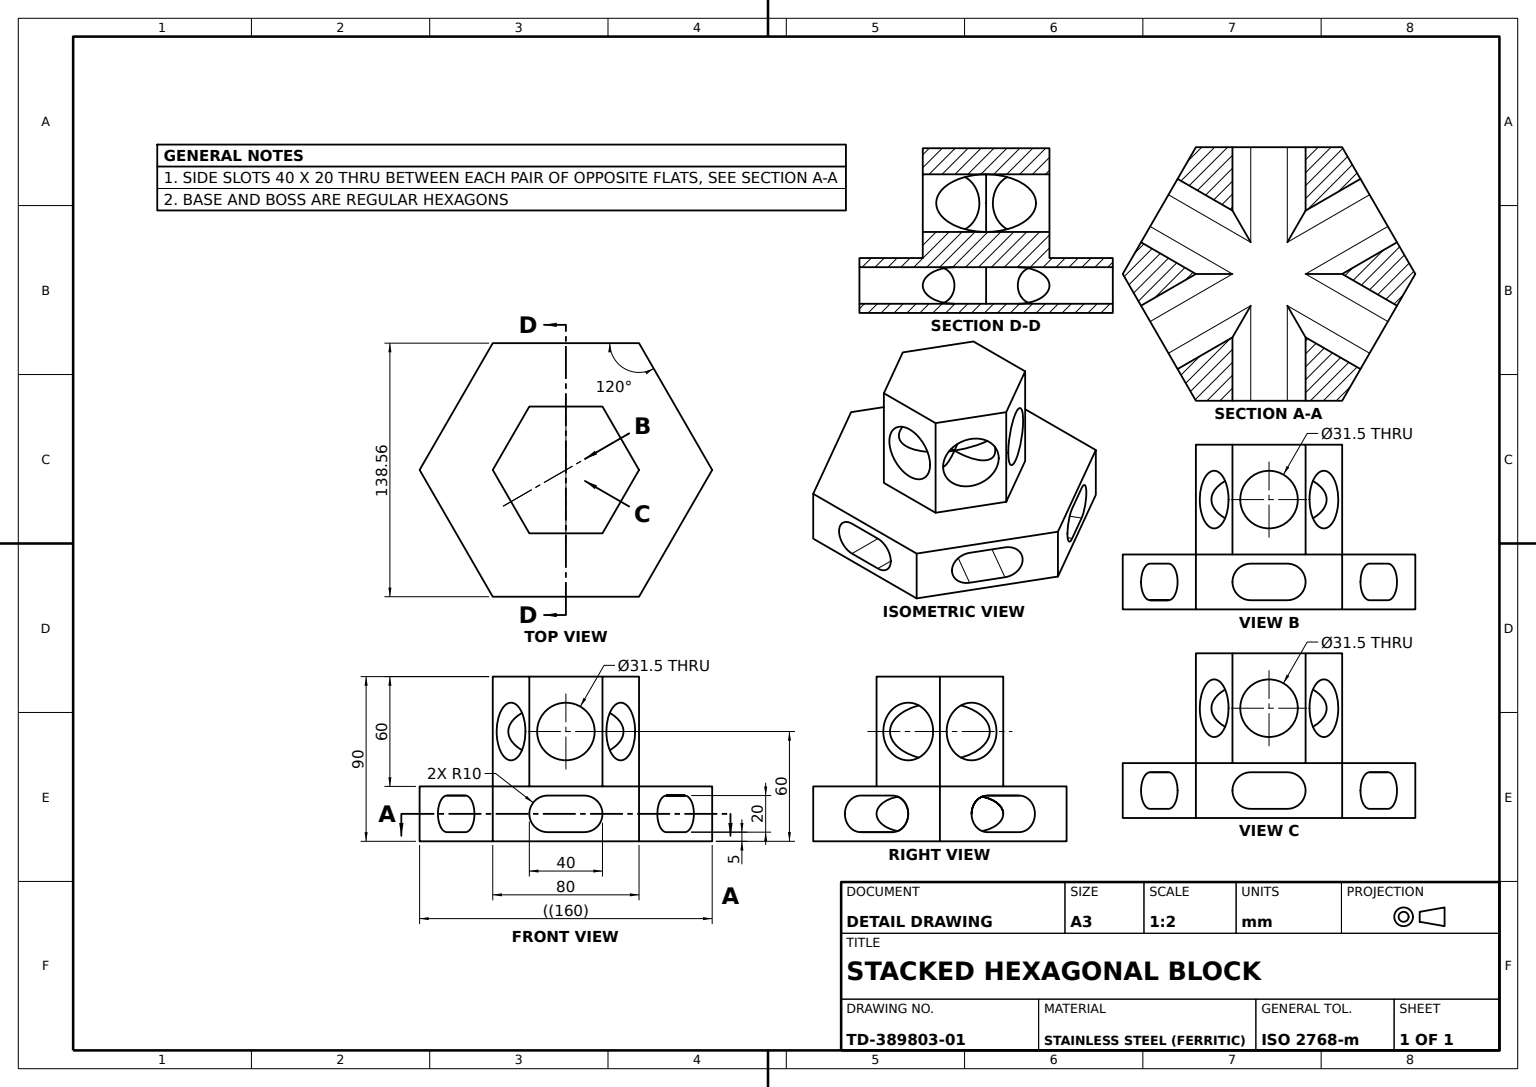
SolidWorks part; units mm, degrees
material "Stainless Steel (ferritic)"
ref_plane "Front Plane" through (0, 0, 0) normal (0, 0, 1) x (1, 0, 0)
ref_plane "Top Plane" through (0, 0, 0) normal (0, 1, 0) x (1, 0, 0)
ref_plane "Right Plane" through (0, 0, 0) normal (1, 0, 0) x (0, 0, -1)
sketch "Hex Base Sketch" plane through (0, 0, 0) normal (0, 1, 0) x (1, 0, 0)
  line L1 (69.282, -40) -> (69.282, 40)
  line L2 (69.282, 40) -> (0, 80)
  line L3 (0, 80) -> (-69.282, 40)
  line L4 (-69.282, 40) -> (-69.282, -40)
  line L5 (-69.282, -40) -> (0, -80)
  line L6 (0, -80) -> (69.282, -40)
  circle A0 centre (0, 0) radius 69.282 construction
  dimension "D1" = 80
extrude "Hex Base" add sketch "Hex Base Sketch" along normal mid plane 30
sketch "Side Slot 1 Sketch" plane through (-69.282, 0, 0) normal (-1, 0, 0) x (0, 0, 1)
  line L0 (-10, 0) -> (10, 0) construction
  line L1 (-10, 10) -> (10, 10)
  line L2 (-10, -10) -> (10, -10)
  arc A0 (-10, 10) -> (-10, -10) centre (-10, 0) ccw
  arc A1 (10, -10) -> (10, 10) centre (10, 0) ccw
  point P2 (0, 0)
  dimension "D2" = 10
  dimension "D1" = 20
extrude "Side Slot 1 20x10" cut sketch "Side Slot 1 Sketch" against normal through all
sketch "Side Slot 2 Sketch" plane through (34.641, 0, -60) normal (0.5, 0, -0.866) x (-0.866, 0, -0.5)
  line L0 (-10, 0) -> (10, 0) construction
  line L1 (-10, 10) -> (10, 10)
  line L2 (-10, -10) -> (10, -10)
  arc A0 (-10, 10) -> (-10, -10) centre (-10, 0) ccw
  arc A1 (10, -10) -> (10, 10) centre (10, 0) ccw
  point P2 (0, 0)
  dimension "D2" = 10
  dimension "D1" = 20
extrude "Side Slot 2 20x10" cut sketch "Side Slot 2 Sketch" against normal through all
sketch "Side Slot 3 Sketch" plane through (-34.641, 0, -60) normal (-0.5, 0, -0.866) x (-0.866, 0, 0.5)
  line L0 (-10, 0) -> (10, 0) construction
  line L1 (-10, 10) -> (10, 10)
  line L2 (-10, -10) -> (10, -10)
  arc A0 (-10, 10) -> (-10, -10) centre (-10, 0) ccw
  arc A1 (10, -10) -> (10, 10) centre (10, 0) ccw
  point P2 (0, 0)
  dimension "D2" = 10
  dimension "D1" = 20
extrude "Side Slot 3 20x10" cut sketch "Side Slot 3 Sketch" against normal through all
sketch "Hex Boss Sketch" plane through (0, 15, 0) normal (0, 1, 0) x (1, 0, 0)
  line L1 (34.641, -20) -> (34.641, 20)
  line L2 (34.641, 20) -> (0, 40)
  line L3 (0, 40) -> (-34.641, 20)
  line L4 (-34.641, 20) -> (-34.641, -20)
  line L5 (-34.641, -20) -> (0, -40)
  line L6 (0, -40) -> (34.641, -20)
  circle A0 centre (0, 0) radius 34.641 construction
  dimension "D1" = 40
extrude "Hex Boss" add sketch "Hex Boss Sketch" along normal blind 60
sketch "Cross Hole 1 Sketch" plane through (34.641, 0, 0) normal (1, 0, 0) x (0, 0, -1)
  line L0 (-20, 75) -> (20, 75) construction
  circle A0 centre (0, 45) radius 15.75
  dimension "D1" = 31.5
  dimension "D2" = 30
extrude "Cross Hole 1 Ø31.5" cut sketch "Cross Hole 1 Sketch" against normal through all
sketch "Cross Hole 2 Sketch" plane through (17.3205, 0, -30) normal (0.5, 0, -0.866) x (-0.866, 0, -0.5)
  circle A0 centre (0, 45) radius 15.75
  dimension "D1" = 31.5
  dimension "D2" = 30
extrude "Cross Hole 2 Ø31.5" cut sketch "Cross Hole 2 Sketch" against normal through all
sketch "Cross Hole 3 Sketch" plane through (17.3205, 0, 30) normal (0.5, 0, 0.866) x (0.866, 0, -0.5)
  line L0 (20, 75) -> (20, 15) construction
  circle A0 centre (0, 45) radius 15.75
  dimension "D1" = 31.5
  dimension "D2" = 30
  dimension "D3" = 20
extrude "Cross Hole 3 Ø31.5" cut sketch "Cross Hole 3 Sketch" against normal through all
